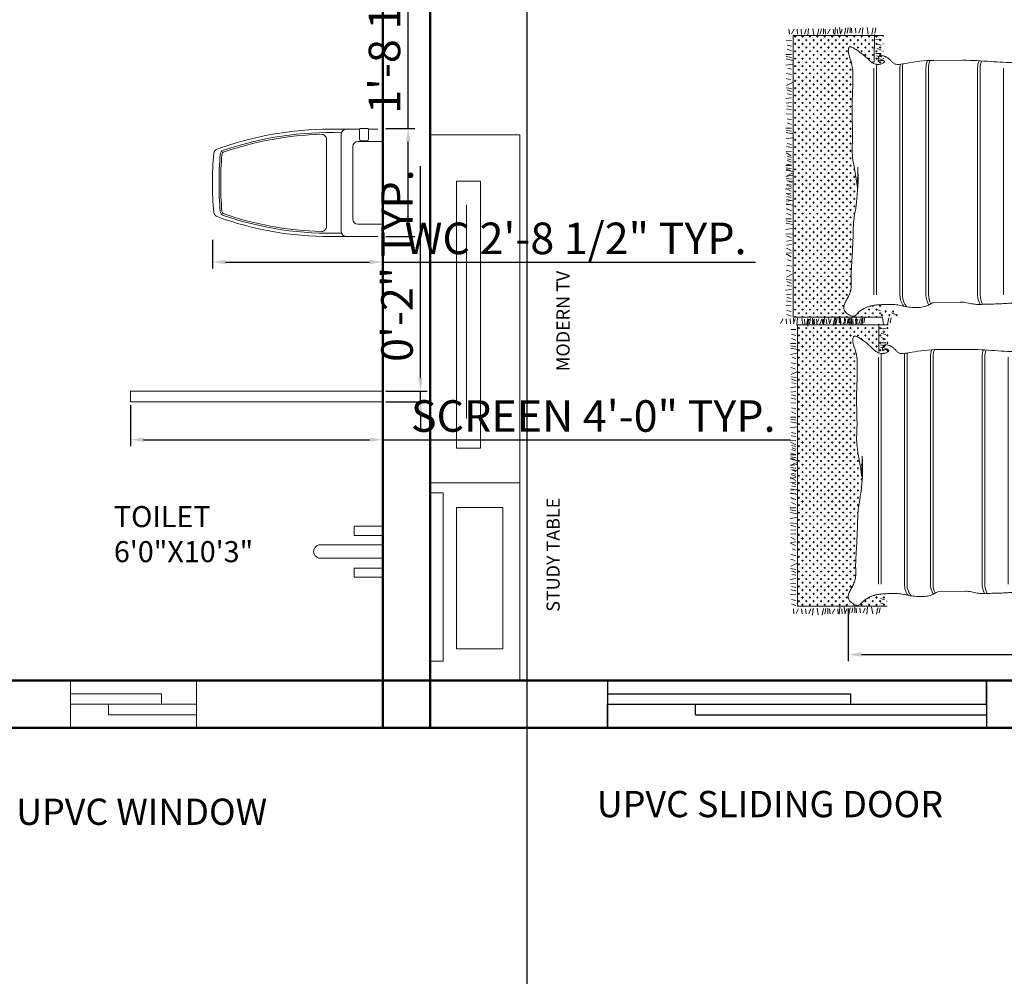
# Model space of a CAD drawing. Units: inches. Extents: x 2123 to 2977, y 1464 to 2698.
# Tile 3 of 10: x 2459 to 2647, y 1923 to 2105. Entities that reach past the tile are written whole.
import ezdxf

# ---------------------------------------------------------------- set-up
doc = ezdxf.new("R2010")
doc.units = ezdxf.units.IN
for name, color, linetype, lineweight in [('A-ANNO-DIMS', 2, 'Continuous', 18), ('A-ANNO-TEXT', 7, 'Continuous', 18), ('A-AREA-IDEN', 7, 'Continuous', 25), ('A-DOOR', 4, 'Continuous', 25), ('A-FLOR-FIXT', 8, 'Continuous', 20), ('A-FURN', 8, 'Continuous', 18), ('A-FURN-FIXD', 8, 'Continuous', 20), ('A-FURN-PATT', 252, 'Continuous', 9), ('A-GLAZ', 4, 'Continuous', 18), ('A-WALL', 7, 'Continuous', 50)]:
    doc.layers.add(name, color=color, linetype=linetype, lineweight=lineweight)
doc.styles.get("Standard").update_dxf_attribs({"font": 'arial.ttf'})
doc.dimstyles.new('ISO-25', dxfattribs={"dimtxt": 6, "dimasz": 2.5, "dimexe": 1.25, "dimexo": 0.625, "dimtad": 1, "dimdec": 0, "dimlunit": 3, "dimtxsty": 'Standard', "dimcen": 2.5, "dimadec": 0, "dimazin": 0, "dimtfac": 1, "dimtdec": 0, "dimtmove": 0, "dimatfit": 3, "dimfxl": 1, "dimarcsym": 0})

# ---------------------------------------------------------------- blocks, each defined once
blk = doc.blocks.new('WC-PLAN')
for p, q in [((27.97, 20.42), (22.38, 20.42)), ((24.5, 19.48), (24.5, 10.21)), ((27.93, 20.26), (27.93, 18.53)), ((29.37, 20.57), (28.24, 20.57)), ((31.41, 20.42), (29.65, 20.42)), ((29.69, 20.26), (29.69, 18.53)), ((32.35, 19.48), (32.35, 10.21)), ((21.67, 18.51), (21.67, 10.21)), ((26.7, 17.12), (26.7, 10.21)), ((32.35, 18.06), (27.64, 18.06)), ((29.37, 18.22), (28.24, 18.22)), ((28.24, 18.22), (28.24, 18.06)), ((29.37, 18.22), (29.37, 18.06)), ((21.67, 1.91), (21.67, 10.21)), ((24.5, 0.94), (24.5, 10.21)), ((26.7, 3.3), (26.7, 10.21)), ((32.35, 0.94), (32.35, 10.21)), ((32.35, 2.36), (27.64, 2.36)), ((31.41, 0), (22.38, 0))]:
    blk.add_line(p, q)
for centre, radius, start, end in [((22.38, -42.41), 62.82, 90, 110.0218), ((22.38, -42.41), 62.2, 88.0034, 109.0034), ((22.38, -42.41), 61.88, 91.5459, 109.0034), ((20.73, 18.51), 0.942, 0, 91.5459), ((25.44, 19.48), 0.942, 90, 180), ((28.24, 20.26), 0.314, 150, 180), ((28.24, 20.26), 0.314, 90, 150), ((29.37, 20.26), 0.314, 30, 90), ((29.37, 20.26), 0.314, 0, 30), ((27.64, 17.12), 0.942, 90, 180), ((28.24, 18.53), 0.314, 180, 270), ((29.37, 18.53), 0.314, 270, 0), ((62.98, 10.21), 62.98, 174.8892, 180), ((1.19, 15.74), 0.942, 110.0218, 174.8892), ((62.98, 10.21), 61.73, 174.9977, 180), ((2.43, 15.51), 0.942, 109.0034, 174.9977), ((62.98, 10.21), 61.41, 174.9977, 180), ((2.43, 15.51), 0.628, 109.0034, 174.9977), ((62.98, 10.21), 62.98, 180, 185.1108), ((62.98, 10.21), 61.73, 180, 185.0023), ((62.98, 10.21), 61.41, 180, 185.0023), ((1.19, 4.68), 0.942, 185.1108, 249.9782), ((22.38, 62.82), 62.82, 249.9782, 270), ((2.43, 4.91), 0.942, 185.0023, 250.9966), ((2.43, 4.91), 0.628, 185.0023, 250.9966), ((22.38, 62.82), 62.2, 250.9966, 271.9966), ((22.38, 62.82), 61.88, 250.9966, 268.4541), ((20.73, 1.91), 0.942, 268.4541, 0), ((27.64, 3.3), 0.942, 180, 270), ((25.44, 0.94), 0.942, 180, 270)]:
    blk.add_arc(centre, radius, start, end)
blk = doc.blocks.new('SHOWER-FITTING')
for points in [[(7.7, 9.7), (13.11, 9.7), (13.11, 7.96), (7.7, 7.96)], [(7.7, 1.74), (13.11, 1.74), (13.11, 0), (7.7, 0)]]:
    blk.add_lwpolyline(points, close=True)
blk.add_lwpolyline([(1, 6.13), (13.11, 6.13), (13.11, 3.63), (1, 3.63)])
blk.add_arc((1.29, 4.88), 1.29, 102.8146, 257.1854)
blk = doc.blocks.new('BED-WITH-PILLOWS')
for p, q in [((5.75, 4.05), (5.75, 47.2)), ((6.24, 4.05), (6.24, 47.2)), ((10.69, 4.05), (10.69, 47.2)), ((11.18, 4.05), (11.18, 47.2)), ((15.63, 4.05), (15.63, 47.2)), ((16.12, 4.05), (16.12, 47.2)), ((25.45, 4.05), (25.45, 47.2)), ((25.94, 4.05), (25.94, 47.2)), ((30.39, 4.05), (30.39, 47.2)), ((33.11, 4.05), (33.11, 47.2)), ((45.27, 2.11), (45.27, 48.58)), ((51.57, 46.51), (45.27, 46.51)), ((51.57, 45.27), (45.27, 45.27)), ((62.41, 46.17), (51.57, 46.17)), ((62.41, 45.03), (51.57, 45.03)), ((51.57, 28.22), (45.27, 28.22)), ((62.41, 5.26), (51.57, 5.26)), ((62.41, 4.13), (51.57, 4.13)), ((62.41, 2.86), (51.57, 2.86))]:
    blk.add_line(p, q)
for points in [[(51.2, 2.51), (50.14, 2.47), (49.31, 2.46), (48.67, 2.48), (48.19, 2.52), (47.84, 2.56), (47.58, 2.61), (47.39, 2.66), (47.22, 2.69), (47.07, 2.7), (46.91, 2.7), (46.77, 2.68), (46.63, 2.65), (46.51, 2.61), (46.41, 2.56), (46.33, 2.52), (46.28, 2.47), (46.26, 2.42), (46.26, 2.38), (46.28, 2.35), (46.3, 2.31), (46.32, 2.28), (46.32, 2.25), (46.31, 2.22), (46.27, 2.2), (46.19, 2.17), (46.08, 2.15), (45.94, 2.13), (45.78, 2.12), (45.61, 2.11), (45.43, 2.1), (45.25, 2.11), (45.07, 2.12), (44.89, 2.14), (44.73, 2.16), (44.57, 2.2), (44.42, 2.24), (44.28, 2.28), (44.15, 2.32), (44.02, 2.37), (43.89, 2.41), (43.77, 2.46), (43.65, 2.5), (43.51, 2.54), (43.35, 2.58), (43.16, 2.62), (42.93, 2.66), (42.65, 2.69), (42.31, 2.72), (41.91, 2.75), (41.46, 2.78), (40.97, 2.8), (40.46, 2.82), (39.94, 2.82), (39.43, 2.83), (38.94, 2.82), (38.48, 2.81), (38.08, 2.78), (37.71, 2.75), (37.37, 2.71), (37.04, 2.67), (36.71, 2.63), (36.37, 2.59), (36, 2.55), (35.6, 2.52), (35.14, 2.5), (34.65, 2.49), (34.14, 2.48), (33.61, 2.47), (33.1, 2.47), (32.6, 2.47), (32.14, 2.47), (31.72, 2.47), (31.37, 2.46), (31.06, 2.45), (30.79, 2.44), (30.55, 2.42), (30.31, 2.41), (30.08, 2.39), (29.82, 2.38), (29.54, 2.36), (29.21, 2.35), (28.86, 2.33), (28.48, 2.32), (28.09, 2.31), (27.69, 2.3), (27.3, 2.29), (26.93, 2.28), (26.58, 2.27), (26.27, 2.26), (25.99, 2.25), (25.73, 2.24), (25.49, 2.24), (25.25, 2.25), (25.02, 2.27), (24.78, 2.29), (24.53, 2.33), (24.27, 2.38), (23.99, 2.44), (23.7, 2.51), (23.41, 2.57), (23.12, 2.62), (22.85, 2.66), (22.59, 2.69), (22.35, 2.68), (22.13, 2.65), (17.06, 2.6), (16.88, 2.53), (16.71, 2.44), (16.54, 2.35), (16.37, 2.25), (16.2, 2.15), (16.01, 2.05), (15.8, 1.96), (15.58, 1.89), (15.34, 1.82), (15.08, 1.77), (14.81, 1.72), (14.53, 1.69), (14.24, 1.67), (13.93, 1.66), (13.62, 1.66), (13.3, 1.67), (12.98, 1.69), (12.67, 1.72), (12.35, 1.75), (12.05, 1.79), (11.76, 1.84), (11.49, 1.89), (11.24, 1.94), (11, 1.99), (10.76, 2.04), (10.52, 2.09), (10.28, 2.14), (10.02, 2.18), (9.74, 2.21), (9.43, 2.24), (9.08, 2.25), (8.71, 2.26), (8.32, 2.26), (7.93, 2.25), (7.53, 2.24), (7.16, 2.22), (6.8, 2.2), (6.49, 2.17), (6.21, 2.15), (5.97, 2.12), (5.77, 2.09), (5.59, 2.06), (5.44, 2.03), (5.3, 2), (5.18, 1.97), (5.07, 1.94), (4.96, 1.91), (4.85, 1.88), (4.74, 1.85), (4.63, 1.81), (4.51, 1.77), (4.39, 1.72), (4.26, 1.67), (4.12, 1.61), (3.98, 1.53), (3.82, 1.46), (3.67, 1.37), (3.51, 1.27), (3.35, 1.17), (3.19, 1.06), (3.04, 0.94), (2.9, 0.81), (2.76, 0.68), (2.64, 0.54), (2.52, 0.41), (2.4, 0.28), (2.28, 0.18), (2.15, 0.09), (2, 0.03), (1.84, 0), (1.67, 0.01), (1.48, 0.05), (1.28, 0.12), (1.09, 0.21), (0.89, 0.33), (0.71, 0.46), (0.54, 0.6), (0.39, 0.74), (0.26, 0.89), (0.17, 1.04), (0.09, 1.19), (0.04, 1.34), (0.01, 1.49), (0, 1.65), (0.01, 1.81), (0.04, 1.97), (0.08, 2.13), (0.14, 2.3), (0.21, 2.47), (0.29, 2.64), (0.38, 2.82), (0.48, 3), (0.58, 3.18), (0.68, 3.37), (0.79, 3.57), (0.9, 3.77), (1, 3.97), (1.09, 4.19), (1.18, 4.41), (1.26, 4.64), (1.32, 4.89), (1.37, 5.14), (1.4, 5.4), (1.42, 5.68), (1.43, 5.97), (1.43, 6.29), (1.42, 6.62), (1.42, 6.98), (1.41, 7.36), (1.41, 7.77), (1.42, 8.21), (1.44, 8.67), (1.46, 9.16), (1.49, 9.65), (1.52, 10.16), (1.55, 10.68), (1.58, 11.19), (1.61, 11.69), (1.64, 12.19), (1.67, 12.67), (1.69, 13.14), (1.72, 13.6), (1.73, 14.05), (1.75, 14.49), (1.77, 14.91), (1.78, 15.32), (1.79, 15.72), (1.79, 16.1), (1.8, 16.48), (1.81, 16.85), (1.83, 17.21), (1.85, 17.56), (1.88, 17.91), (1.91, 18.25), (1.96, 18.58), (2.01, 18.93), (2.07, 19.29), (2.14, 19.68), (2.21, 20.11), (2.29, 20.58), (2.36, 21.11), (2.44, 21.71), (2.51, 22.39), (2.58, 23.13), (2.64, 23.92), (2.69, 24.77), (2.72, 25.64), (2.73, 26.54), (2.71, 27.44), (2.67, 28.35), (2.59, 24.41), (2.49, 25.28), (2.37, 26.12), (2.24, 26.93), (2.11, 27.7), (1.98, 28.42), (1.86, 29.08), (1.76, 29.68), (1.69, 30.2), (1.64, 30.67), (1.61, 31.08), (1.59, 31.44), (1.59, 31.77), (1.6, 32.08), (1.61, 32.36), (1.63, 32.64), (1.64, 32.92), (1.66, 33.21), (1.67, 33.51), (1.67, 33.82), (1.68, 34.16), (1.68, 34.52), (1.68, 34.92), (1.67, 35.35), (1.66, 35.83), (1.64, 36.35), (1.62, 36.91), (1.61, 37.51), (1.6, 38.16), (1.59, 38.85), (1.59, 39.57), (1.6, 40.34), (1.62, 41.15), (1.65, 41.98), (1.68, 42.82), (1.7, 43.65), (1.72, 44.46), (1.73, 45.24), (1.72, 45.95), (1.7, 46.6), (1.64, 47.17), (1.57, 47.65), (1.48, 48.08), (1.39, 48.45), (1.29, 48.77), (1.19, 49.06), (1.1, 49.32), (1.02, 49.57), (0.96, 49.81), (0.91, 50.04), (0.89, 50.26), (0.87, 50.46), (0.88, 50.65), (0.9, 50.81), (0.93, 50.95), (0.98, 51.06), (1.04, 51.14), (1.12, 51.2), (1.21, 51.22), (1.31, 51.22), (1.43, 51.19), (1.55, 51.15), (1.69, 51.09), (1.84, 51.01), (2.01, 50.92), (2.18, 50.81), (2.36, 50.7), (2.54, 50.57), (2.72, 50.45), (2.91, 50.31), (3.09, 50.18), (3.27, 50.04), (3.45, 49.9), (3.62, 49.77), (3.78, 49.63), (3.93, 49.5), (4.08, 49.37), (4.23, 49.24), (4.37, 49.11), (4.5, 48.99), (4.63, 48.86), (4.76, 48.74), (4.88, 48.62), (5.01, 48.5), (5.14, 48.4), (5.27, 48.3), (5.41, 48.2), (5.55, 48.12), (5.71, 48.05), (5.87, 48), (6.04, 47.95), (6.22, 47.92), (6.39, 47.9), (6.56, 47.89), (6.73, 47.9), (6.89, 47.92), (7.04, 47.96), (7.18, 48.01), (7.31, 48.07), (7.43, 48.13), (7.53, 48.2), (7.61, 48.27), (7.67, 48.33), (7.71, 48.39), (7.73, 48.44), (7.73, 48.49), (7.71, 48.52), (7.68, 48.55), (7.63, 48.58), (7.56, 48.6), (7.49, 48.61), (7.42, 48.62), (7.33, 48.63), (7.25, 48.64), (7.16, 48.64), (7.07, 48.64), (6.99, 48.63), (6.91, 48.62), (6.83, 48.6), (6.77, 48.58), (6.71, 48.55), (6.67, 48.52), (6.63, 48.5), (6.6, 48.47), (6.57, 48.46), (6.56, 48.46), (6.55, 48.48), (6.54, 48.51), (6.54, 48.58)], [(6.54, 48.66), (6.54, 48.76), (6.55, 48.86), (6.56, 48.97), (6.58, 49.08), (6.61, 49.18), (6.63, 49.27), (6.67, 49.34), (6.7, 49.4), (6.75, 49.44), (6.79, 49.47), (6.84, 49.5), (6.9, 49.51), (6.95, 49.52), (7.01, 49.53), (7.07, 49.53), (7.14, 49.53), (7.21, 49.53), (7.28, 49.53), (7.35, 49.53), (7.43, 49.52), (7.51, 49.5), (7.59, 49.49), (7.68, 49.46), (7.77, 49.43), (7.86, 49.4), (7.96, 49.36), (8.06, 49.31), (8.16, 49.26), (8.27, 49.19), (8.37, 49.12), (8.48, 49.04), (8.59, 48.95), (8.69, 48.86), (8.8, 48.76), (8.9, 48.66), (9.01, 48.56), (9.1, 48.45), (9.2, 48.35), (9.29, 48.25), (9.38, 48.16), (9.48, 48.07), (9.61, 48), (9.76, 47.94), (9.95, 47.91), (10.18, 47.89), (10.46, 47.89), (10.81, 47.93), (11.21, 47.98), (11.65, 48.06), (12.15, 48.14), (12.68, 48.23), (13.25, 48.32), (13.84, 48.41), (14.46, 48.49), (15.09, 48.55), (15.74, 48.6), (16.41, 48.64), (17.08, 48.66), (22.63, 48.67), (23.31, 48.67), (23.98, 48.66), (24.65, 48.64), (25.32, 48.61), (25.97, 48.57), (26.62, 48.53), (27.26, 48.49), (27.89, 48.44), (28.51, 48.4), (29.12, 48.36), (29.71, 48.33), (30.3, 48.3), (30.87, 48.28), (31.43, 48.27), (31.97, 48.28), (32.5, 48.29), (33, 48.32), (33.49, 48.36), (33.95, 48.42), (34.39, 48.49), (34.81, 48.58), (35.23, 48.67), (35.64, 48.77), (36.07, 48.87), (36.5, 48.96), (36.96, 49.05), (37.46, 49.12), (37.99, 49.18), (38.55, 49.22), (39.13, 49.24), (39.73, 49.25), (40.33, 49.24), (40.93, 49.22), (41.52, 49.18), (42.1, 49.12), (42.65, 49.05), (43.17, 48.96), (43.66, 48.87), (44.14, 48.78), (44.58, 48.7), (45, 48.62), (45.4, 48.56), (45.77, 48.51), (46.12, 48.5), (46.45, 48.5), (46.77, 48.51), (47.08, 48.53), (47.4, 48.56), (47.73, 48.57), (48.08, 48.58), (48.45, 48.58), (48.84, 48.55), (49.25, 48.49), (49.68, 48.41), (50.1, 48.3), (50.5, 48.16), (50.88, 47.98), (51.23, 47.77), (51.53, 47.52)], [(51.57, 47.43), (51.57, 2.81), (45.27, 2.81)], [(51.57, 47.43), (62.41, 47.43)], [(45.27, 43.15), (51.57, 43.15)], [(51.57, 41.91), (45.27, 41.91)], [(45.27, 39.44), (51.57, 39.44)], [(51.57, 38.2), (45.27, 38.2)], [(45.27, 35.73), (51.57, 35.73)], [(51.57, 34.5), (45.27, 34.5)], [(45.27, 32.03), (51.57, 32.03)], [(51.57, 30.79), (45.27, 30.79)], [(45.27, 28.32), (51.57, 28.32)], [(51.57, 27.09), (45.27, 27.09)], [(45.27, 25.74), (51.57, 25.74)], [(45.27, 24.62), (51.57, 24.62)], [(51.57, 24.51), (45.27, 24.51)], [(51.57, 23.38), (45.27, 23.38)], [(45.27, 22.04), (51.57, 22.04)], [(51.57, 20.8), (45.27, 20.8)], [(45.27, 18.33), (51.57, 18.33)], [(51.57, 17.1), (45.27, 17.1)], [(45.27, 14.63), (51.57, 14.63)], [(51.57, 13.39), (45.27, 13.39)], [(45.27, 10.92), (51.57, 10.92)], [(51.57, 9.69), (45.27, 9.69)], [(45.27, 7.22), (51.57, 7.22)], [(51.57, 5.98), (45.27, 5.98)], [(45.27, 4.05), (51.57, 4.05)]]:
    blk.add_lwpolyline(points)
blk.add_lwpolyline([(51.57, 46.51), (51.57, 45.27), (45.27, 45.27), (45.27, 46.51)], close=True)
for centre, radius, start, end in [((9.74, 47.23), 3.5, 168.8455, 180.4575), ((14.19, 47.23), 3.5, 168.5644, 180.4575), ((14.68, 47.23), 3.5, 167.3874, 180.4575), ((19.13, 47.23), 3.5, 156.778, 180.4575), ((19.62, 47.23), 3.5, 156.3002, 180.4575), ((28.95, 47.23), 3.5, 157.2176, 180.4575), ((29.45, 47.23), 3.5, 157.7219, 180.4575), ((36.12, 47.23), 3.5, 162.3249, 180.4575), ((36.61, 47.23), 3.5, 162.5343, 180.4575), ((113.8, 36.55), 60.42, 176.9417, 187.4263), ((56.43, 21.05), 18.95, 81.0114, 98.9886), ((56.69, 54.69), 15.26, 257.8171, 275.8068), ((60.35, 32.94), 6.89, 82.0225, 107.8578), ((-19.09, 32.85), 80.7, 355.082, 4.918), ((33.93, 30.3), 20.02, 347.406, 13.4182), ((55.08, 36.57), 10.76, 261.3968, 285.5408), ((59.18, 20.45), 5.88, 68.7829, 101.9106), ((59.54, 25.52), 1.81, 13.0862, 85.1007), ((113.8, 22.01), 60.42, 176.9417, 187.4263), ((56.43, 6.52), 18.95, 81.0114, 98.9886), ((56.69, 40.15), 15.26, 257.8171, 275.8068), ((59.11, 48.58), 22.76, 264.4677, 275.5323), ((60.35, 18.41), 6.89, 82.0225, 107.8578), ((-19.09, 18.32), 80.7, 355.082, 4.918), ((33.93, 15.76), 20.02, 347.406, 13.4182), ((55.08, 22.03), 10.76, 261.3968, 285.5408), ((59.11, 34.05), 22.76, 264.4677, 275.5323), ((59.18, 5.91), 5.88, 68.7829, 101.9106), ((59.54, 10.99), 1.81, 13.0862, 85.1007), ((14.19, 4.02), 3.5, 179.5425, 217.0761), ((14.68, 4.02), 3.5, 179.5425, 219.1707), ((19.13, 4.02), 3.5, 179.5425, 212.5319), ((19.62, 4.02), 3.5, 179.5425, 208.4654), ((28.95, 4.02), 3.5, 179.5425, 210.3906), ((29.45, 4.02), 3.5, 179.5425, 210.1306), ((36.12, 4.02), 3.5, 179.5425, 206.8424), ((36.61, 4.02), 3.5, 179.5425, 206.471)]:
    blk.add_arc(centre, radius, start, end)
blk = doc.blocks.new('SHOWER-SCREEN')
for p, q in [((47.94, 2), (0, 2)), ((0, 2), (0, 0)), ((0, 0), (47.94, 0))]:
    blk.add_line(p, q)
blk = doc.blocks.new('*D42')
at = {"layer": 'A-ANNO-DIMS', "color": 0, "lineweight": -2, "transparency": 16777216}
for p, q in [((2496.08, 2062.68), (2496.08, 2057.2)), ((2528.44, 2062.68), (2528.44, 2057.2)), ((2498.58, 2058.45), (2525.94, 2058.45)), ((2528.44, 2058.45), (2599.28, 2058.45))]:
    blk.add_line(p, q, dxfattribs=at)
at = {"layer": 'A-ANNO-DIMS', "color": 0, "transparency": 16777216}
for points in [[(2498.58, 2058.87), (2498.58, 2058.03), (2496.08, 2058.45)], [(2525.94, 2058.87), (2525.94, 2058.03), (2528.44, 2058.45)]]:
    blk.add_solid(points, dxfattribs=at)
at = {"layer": 'Defpoints', "color": 0, "transparency": 16777216}
for p in [(2496.08, 2063.3), (2528.44, 2063.3), (2528.44, 2058.45)]:
    blk.add_point(p, dxfattribs=at)
at = {"layer": 'A-ANNO-DIMS', "color": 0, "transparency": 16777216, "insert": (2565.11, 2062.18), "char_height": 6, "attachment_point": 5}
blk.add_mtext('WC 2\'-8 1/2" TYP.', dxfattribs=at)
blk = doc.blocks.new('*D43')
at = {"layer": 'A-ANNO-DIMS', "color": 0, "lineweight": -2, "transparency": 16777216}
for p, q in [((2533.29, 2083.88), (2533.29, 2137.62)), ((2529.06, 2083.88), (2534.54, 2083.88)), ((2533.29, 2065.8), (2533.29, 2081.38)), ((2529.06, 2063.3), (2534.54, 2063.3))]:
    blk.add_line(p, q, dxfattribs=at)
at = {"layer": 'A-ANNO-DIMS', "color": 0, "transparency": 16777216}
for points in [[(2532.87, 2081.38), (2533.71, 2081.38), (2533.29, 2083.88)], [(2532.87, 2065.8), (2533.71, 2065.8), (2533.29, 2063.3)]]:
    blk.add_solid(points, dxfattribs=at)
at = {"layer": 'Defpoints', "color": 0, "transparency": 16777216}
for p in [(2528.44, 2083.88), (2533.29, 2083.88), (2528.44, 2063.3)]:
    blk.add_point(p, dxfattribs=at)
at = {"layer": 'A-ANNO-DIMS', "color": 0, "transparency": 16777216, "insert": (2529.56, 2112), "char_height": 6, "attachment_point": 5, "rotation": 90}
blk.add_mtext('1\'-8 1/2" TYP.', dxfattribs=at)
blk = doc.blocks.new('*D48')
at = {"layer": 'A-ANNO-DIMS', "color": 0, "lineweight": -2, "transparency": 16777216}
for p, q in [((2616.93, 1992.55), (2616.93, 1982.56)), ((2679.35, 1992.55), (2679.35, 1982.56)), ((2619.43, 1983.81), (2676.85, 1983.81)), ((2679.35, 1983.81), (2752.95, 1983.81))]:
    blk.add_line(p, q, dxfattribs=at)
at = {"layer": 'A-ANNO-DIMS', "color": 0, "transparency": 16777216}
for points in [[(2619.43, 1984.23), (2619.43, 1983.39), (2616.93, 1983.81)], [(2676.85, 1984.23), (2676.85, 1983.39), (2679.35, 1983.81)]]:
    blk.add_solid(points, dxfattribs=at)
at = {"layer": 'Defpoints', "color": 0, "transparency": 16777216}
for p in [(2616.93, 1993.17), (2679.35, 1993.17), (2679.35, 1983.81)]:
    blk.add_point(p, dxfattribs=at)
at = {"layer": 'A-ANNO-DIMS', "color": 0, "transparency": 16777216, "insert": (2717.4, 1987.54), "char_height": 6, "attachment_point": 5}
blk.add_mtext('BED 5\'-2 1/2" TYP.', dxfattribs=at)
blk = doc.blocks.new('*D52')
at = {"layer": 'A-ANNO-DIMS', "color": 0, "lineweight": -2, "transparency": 16777216}
for p, q in [((2480.5, 2031.24), (2480.5, 2023.42)), ((2528.44, 2031.24), (2528.44, 2023.42)), ((2483, 2024.67), (2525.94, 2024.67)), ((2528.44, 2024.67), (2605.99, 2024.67))]:
    blk.add_line(p, q, dxfattribs=at)
at = {"layer": 'A-ANNO-DIMS', "color": 0, "transparency": 16777216}
for points in [[(2483, 2025.09), (2483, 2024.26), (2480.5, 2024.67)], [(2525.94, 2025.09), (2525.94, 2024.26), (2528.44, 2024.67)]]:
    blk.add_solid(points, dxfattribs=at)
at = {"layer": 'Defpoints', "color": 0, "transparency": 16777216}
for p in [(2480.5, 2031.87), (2528.44, 2031.87), (2528.44, 2024.67)]:
    blk.add_point(p, dxfattribs=at)
at = {"layer": 'A-ANNO-DIMS', "color": 0, "transparency": 16777216, "insert": (2568.46, 2028.4), "char_height": 6, "attachment_point": 5}
blk.add_mtext('SCREEN 4\'-0" TYP.', dxfattribs=at)
blk = doc.blocks.new('*D53')
at = {"layer": 'A-ANNO-DIMS', "color": 0, "lineweight": -2, "transparency": 16777216}
for p, q in [((2535.63, 2036.37), (2535.63, 2076.69)), ((2529.06, 2033.87), (2536.88, 2033.87)), ((2535.63, 2031.87), (2535.63, 2033.87)), ((2529.06, 2031.87), (2536.88, 2031.87)), ((2535.63, 2029.37), (2535.63, 2026.87))]:
    blk.add_line(p, q, dxfattribs=at)
at = {"layer": 'A-ANNO-DIMS', "color": 0, "transparency": 16777216}
for points in [[(2535.21, 2036.37), (2536.04, 2036.37), (2535.63, 2033.87)], [(2535.21, 2029.37), (2536.04, 2029.37), (2535.63, 2031.87)]]:
    blk.add_solid(points, dxfattribs=at)
at = {"layer": 'Defpoints', "color": 0, "transparency": 16777216}
for p in [(2528.44, 2033.87), (2535.63, 2033.87), (2528.44, 2031.87)]:
    blk.add_point(p, dxfattribs=at)
at = {"layer": 'A-ANNO-DIMS', "color": 0, "transparency": 16777216, "insert": (2531.94, 2057.78), "char_height": 6, "attachment_point": 5, "rotation": 90}
blk.add_mtext('0\'-2" TYP.', dxfattribs=at)
blk = doc.blocks.new('*D57')
at = {"layer": 'A-ANNO-DIMS', "color": 0, "lineweight": -2, "transparency": 16777216}
for p, q in [((2555.89, 1805.13), (2555.89, 2606.82)), ((2558.39, 2605.57), (2755.44, 2605.57)), ((2757.94, 1805.13), (2757.94, 2606.82))]:
    blk.add_line(p, q, dxfattribs=at)
at = {"layer": 'A-ANNO-DIMS', "color": 0, "transparency": 16777216}
for points in [[(2558.39, 2605.99), (2558.39, 2605.15), (2555.89, 2605.57)], [(2755.44, 2605.99), (2755.44, 2605.15), (2757.94, 2605.57)]]:
    blk.add_solid(points, dxfattribs=at)
at = {"layer": 'Defpoints', "color": 0, "transparency": 16777216}
for p in [(2757.94, 2605.57), (2555.89, 1804.5), (2757.94, 1804.5)]:
    blk.add_point(p, dxfattribs=at)
at = {"layer": 'A-ANNO-DIMS', "color": 0, "transparency": 16777216, "insert": (2656.91, 2609.26), "char_height": 6, "attachment_point": 5}
blk.add_mtext('16\'-10"', dxfattribs=at)

msp = doc.modelspace()

# ---------------------------------------------------------------- hatches: boundary and pattern name
at = {"layer": 'A-FURN-PATT'}
h = msp.add_hatch(dxfattribs=at)
h.set_pattern_fill('CROSS', color=256, scale=0.1105279, style=0)
h.paths.add_polyline_path([(2606.45, 2047.98), (2623.47, 2047.98), (2623.47, 2050.38), (2623.23, 2050.37), (2622.28, 2050.3), (2621.66, 2050.22), (2621.26, 2050.13), (2620.92, 2050.03), (2620.59, 2049.92), (2620.2, 2049.76), (2619.74, 2049.52), (2619.26, 2049.21), (2618.84, 2048.83), (2618.48, 2048.44), (2618.08, 2048.18), (2617.56, 2048.2), (2616.97, 2048.48), (2616.46, 2048.9), (2616.17, 2049.34), (2616.08, 2049.81), (2616.15, 2050.29), (2616.36, 2050.79), (2616.65, 2051.34), (2616.97, 2051.92), (2617.26, 2052.57), (2617.45, 2053.29), (2617.5, 2054.13), (2617.49, 2055.13), (2617.5, 2056.36), (2617.56, 2057.81), (2617.66, 2059.34), (2617.75, 2060.83), (2617.81, 2062.2), (2617.85, 2063.47), (2617.88, 2064.64), (2617.92, 2065.71), (2618.03, 2066.74), (2618.21, 2067.84), (2618.44, 2069.27), (2618.66, 2071.28), (2618.79, 2073.8), (2618.74, 2076.5), (2618.45, 2074.28), (2618.05, 2076.57), (2617.77, 2078.36), (2617.67, 2079.6), (2617.69, 2080.52), (2617.73, 2081.36), (2617.75, 2082.31), (2617.74, 2083.51), (2617.7, 2085.06), (2617.67, 2087), (2617.7, 2089.3), (2617.78, 2091.81), (2617.8, 2094.11), (2617.65, 2095.81), (2617.36, 2096.92), (2617.1, 2097.72), (2616.96, 2098.41), (2616.97, 2098.97), (2617.12, 2099.3), (2617.39, 2099.37), (2617.77, 2099.24), (2618.25, 2098.97), (2618.8, 2098.6), (2619.35, 2098.19), (2619.85, 2097.79), (2620.3, 2097.4), (2620.71, 2097.02), (2621.08, 2096.66), (2621.48, 2096.36), (2621.95, 2096.15), (2622.47, 2096.05), (2622.97, 2096.08), (2623.39, 2096.22), (2623.65, 2096.4), (2623.65, 2101.52), (2606.45, 2101.52)])
h = msp.add_hatch(dxfattribs=at)
h.set_pattern_fill('CROSS', color=256, scale=0.1105279, style=0)
h.paths.add_polyline_path([(2607.31, 1993), (2624.33, 1993), (2624.33, 1995.4), (2624.09, 1995.39), (2623.14, 1995.32), (2622.52, 1995.23), (2622.11, 1995.14), (2621.78, 1995.05), (2621.44, 1994.94), (2621.06, 1994.78), (2620.6, 1994.54), (2620.12, 1994.23), (2619.7, 1993.85), (2619.33, 1993.46), (2618.94, 1993.2), (2618.41, 1993.22), (2617.82, 1993.5), (2617.32, 1993.91), (2617.02, 1994.36), (2616.93, 1994.82), (2617.01, 1995.3), (2617.22, 1995.81), (2617.51, 1996.35), (2617.83, 1996.94), (2618.11, 1997.58), (2618.3, 1998.31), (2618.36, 1999.15), (2618.35, 2000.15), (2618.35, 2001.38), (2618.42, 2002.83), (2618.52, 2004.36), (2618.6, 2005.84), (2618.67, 2007.22), (2618.71, 2008.49), (2618.74, 2009.65), (2618.78, 2010.73), (2618.89, 2011.76), (2619.07, 2012.85), (2619.29, 2014.28), (2619.51, 2016.3), (2619.65, 2018.81), (2619.6, 2021.52), (2619.3, 2019.29), (2618.91, 2021.59), (2618.62, 2023.37), (2618.53, 2024.61), (2618.55, 2025.54), (2618.59, 2026.38), (2618.61, 2027.33), (2618.6, 2028.52), (2618.56, 2030.08), (2618.52, 2032.02), (2618.55, 2034.32), (2618.64, 2036.82), (2618.66, 2039.12), (2618.5, 2040.83), (2618.22, 2041.94), (2617.95, 2042.74), (2617.82, 2043.43), (2617.83, 2043.98), (2617.98, 2044.32), (2618.24, 2044.39), (2618.63, 2044.26), (2619.11, 2043.98), (2619.66, 2043.62), (2620.21, 2043.21), (2620.71, 2042.81), (2621.16, 2042.41), (2621.56, 2042.03), (2621.94, 2041.68), (2622.34, 2041.38), (2622.81, 2041.17), (2623.32, 2041.07), (2623.82, 2041.09), (2624.25, 2041.24), (2624.51, 2041.41), (2624.51, 2046.54), (2607.31, 2046.54)])

# ---------------------------------------------------------------- linework, layer by layer
at = {"layer": 'A-DOOR'}
for p, q in [((2571.19, 1978.87), (2571.19, 1969.87)), ((2643.19, 1974.37), (2643.19, 1978.87)), ((2643.19, 1978.87), (2643.19, 1969.87)), ((2571.19, 1976.37), (2617.34, 1976.37)), ((2617.34, 1976.37), (2617.34, 1974.37)), ((2571.19, 1969.87), (2571.19, 1974.37)), ((2571.19, 1974.37), (2643.19, 1974.37)), ((2587.91, 1972.37), (2587.91, 1974.37)), ((2587.91, 1972.37), (2643.19, 1972.37))]:
    msp.add_line(p, q, dxfattribs=at)
at = {"layer": 'A-FURN'}
for p, q in [((2605.67, 2102.74), (2605.76, 2101.8)), ((2606.64, 2102.74), (2606.16, 2101.88)), ((2607.23, 2102.74), (2607.32, 2101.8)), ((2607.98, 2102.74), (2608.07, 2101.8)), ((2608.95, 2102.74), (2608.6, 2101.8)), ((2609.39, 2102.89), (2609.26, 2101.57)), ((2610.18, 2102.89), (2610.38, 2101.64)), ((2611.37, 2102.82), (2611.1, 2101.57)), ((2611.83, 2102.82), (2611.63, 2101.8)), ((2612.22, 2102.89), (2612.22, 2101.84)), ((2612.52, 2102.74), (2612.61, 2101.8)), ((2613.5, 2102.74), (2613.01, 2101.88)), ((2614.08, 2102.74), (2614.17, 2101.8)), ((2614.49, 2103.07), (2614.36, 2101.74)), ((2614.83, 2102.74), (2614.93, 2101.8)), ((2615.28, 2103.07), (2615.48, 2101.82)), ((2615.81, 2102.74), (2615.45, 2101.8)), ((2616.47, 2102.99), (2616.2, 2101.74)), ((2616.93, 2102.99), (2616.74, 2101.98)), ((2617.32, 2103.07), (2617.32, 2102.02)), ((2617.56, 2102.92), (2617.65, 2101.98)), ((2618.32, 2102.92), (2618.41, 2101.98)), ((2619.29, 2102.92), (2618.93, 2101.98)), ((2619.72, 2103.07), (2619.6, 2101.74)), ((2620.52, 2103.07), (2620.72, 2101.82)), ((2621.7, 2102.99), (2621.44, 2101.74)), ((2622.16, 2102.99), (2621.97, 2101.98)), ((2605.15, 2100.63), (2606.13, 2100.58)), ((2606.45, 2047.98), (2606.45, 2101.52)), ((2606.45, 2101.52), (2623.65, 2101.52)), ((2621.9, 2101.7), (2621.87, 2096.45)), ((2622.21, 2100.81), (2623.2, 2100.76)), ((2605.3, 2099.71), (2606.13, 2099.49)), ((2605.3, 2098.92), (2606.13, 2098.59)), ((2622.15, 2098.1), (2623.2, 2098.1)), ((2622.36, 2099.89), (2623.2, 2099.67)), ((2622.36, 2099.1), (2623.2, 2098.77)), ((2605.08, 2097.93), (2606.13, 2097.93)), ((2605.16, 2097.53), (2606.17, 2097.34)), ((2605.16, 2097.07), (2606.41, 2096.8)), ((2622.22, 2097.7), (2623.24, 2097.51)), ((2622.22, 2097.24), (2623.47, 2096.98)), ((2605.08, 2095.88), (2606.33, 2096.09)), ((2605.45, 2095.35), (2606.13, 2095.12)), ((2605.15, 2093.37), (2606.01, 2093.11)), ((2605.22, 2092.05), (2606.32, 2092.58)), ((2605.23, 2094.31), (2606.16, 2094.1)), ((2605.15, 2091.59), (2606.17, 2091.46)), ((2605.3, 2091.19), (2606.17, 2090.86)), ((2605.07, 2089.54), (2606.13, 2089.7)), ((2605.15, 2088.69), (2606.13, 2088.82)), ((2605.37, 2090.47), (2606.17, 2090.33)), ((2605.22, 2087.56), (2606.13, 2087.38)), ((2605.3, 2088.16), (2606.13, 2087.97)), ((2605.15, 2086.64), (2606.13, 2086.59)), ((2605.3, 2085.72), (2606.13, 2085.5)), ((2605.08, 2083.94), (2606.13, 2083.94)), ((2605.16, 2083.54), (2606.17, 2083.35)), ((2605.16, 2083.08), (2606.41, 2082.81)), ((2605.3, 2084.93), (2606.13, 2084.61)), ((2605.08, 2081.89), (2606.33, 2082.1)), ((2605.15, 2079.49), (2606.13, 2079.44)), ((2605.22, 2080.41), (2606.13, 2080.23)), ((2605.3, 2081.01), (2606.13, 2080.82)), ((2605.11, 2079.21), (2606.1, 2078.66)), ((2605.3, 2078.57), (2606.13, 2078.35)), ((2605.3, 2077.78), (2606.13, 2077.46)), ((2605.41, 2078.1), (2606.1, 2077.87)), ((2605.08, 2076.79), (2606.13, 2076.79)), ((2605.11, 2076.13), (2605.98, 2075.86)), ((2605.16, 2076.39), (2606.17, 2076.2)), ((2605.16, 2075.93), (2606.41, 2075.66)), ((2605.2, 2077.06), (2606.13, 2076.85)), ((2605.08, 2074.74), (2606.33, 2074.95)), ((2605.11, 2074.34), (2606.14, 2074.21)), ((2605.19, 2074.8), (2606.29, 2075.33)), ((2605.26, 2073.94), (2606.14, 2073.61)), ((2605.56, 2073.9), (2606.36, 2073.72)), ((2605.04, 2072.3), (2606.1, 2072.45)), ((2605.11, 2072.47), (2606.1, 2071.92)), ((2605.2, 2073.11), (2606.14, 2072.67)), ((2605.34, 2073.23), (2606.14, 2073.09)), ((2605.11, 2071.44), (2606.1, 2071.57)), ((2605.11, 2070.05), (2606.29, 2070.18)), ((2605.19, 2070.32), (2606.1, 2070.13)), ((2605.26, 2070.92), (2606.1, 2070.73)), ((2605.41, 2071.37), (2606.1, 2071.13)), ((2605.11, 2069.4), (2606.1, 2069.35)), ((2605.19, 2069.53), (2606.36, 2069.26)), ((2605.2, 2068.65), (2606.14, 2068.21)), ((2605.26, 2068.48), (2606.1, 2068.25)), ((2605.05, 2066.69), (2606.1, 2066.69)), ((2605.12, 2066.29), (2606.14, 2066.1)), ((2605.26, 2067.68), (2606.1, 2067.36)), ((2605.05, 2064.65), (2606.3, 2064.85)), ((2605.12, 2065.83), (2606.37, 2065.57)), ((2605.05, 2063.85), (2606.37, 2063.73)), ((2605.2, 2063.42), (2606.14, 2063.06)), ((2605.2, 2062.45), (2606.14, 2062.54)), ((2605.2, 2061.69), (2606.14, 2061.78)), ((2605.2, 2061.11), (2606.06, 2060.62)), ((2605.11, 2060), (2606.1, 2059.45)), ((2605.2, 2060.13), (2606.14, 2060.22)), ((2605.41, 2058.9), (2606.1, 2058.66)), ((2605.11, 2056.92), (2605.98, 2056.65)), ((2605.2, 2057.85), (2606.13, 2057.65)), ((2605.11, 2055.13), (2606.14, 2055)), ((2605.19, 2055.59), (2606.29, 2056.13)), ((2605.04, 2053.09), (2606.1, 2053.24)), ((2605.26, 2054.74), (2606.14, 2054.4)), ((2605.34, 2054.02), (2606.14, 2053.88)), ((2605.11, 2052.23), (2606.1, 2052.37)), ((2605.26, 2051.71), (2606.1, 2051.52)), ((2605.11, 2050.19), (2606.1, 2050.14)), ((2605.19, 2051.11), (2606.1, 2050.92)), ((2622.2, 2049.44), (2623.04, 2049.22)), ((2604.56, 2047.63), (2604.07, 2046.76)), ((2605.14, 2047.63), (2605.23, 2046.69)), ((2605.26, 2049.27), (2606.1, 2049.05)), ((2605.26, 2048.48), (2606.1, 2048.15)), ((2605.89, 2047.63), (2605.98, 2046.69)), ((2623.47, 2047.98), (2606.45, 2047.98)), ((2606.87, 2047.63), (2606.51, 2046.69)), ((2606.52, 2047.76), (2606.62, 2046.82)), ((2607.3, 2047.78), (2607.17, 2046.45)), ((2608.09, 2047.78), (2608.29, 2046.53)), ((2608.61, 2047.6), (2608.7, 2046.66)), ((2609.28, 2047.7), (2609.01, 2046.45)), ((2609.59, 2047.6), (2609.1, 2046.73)), ((2609.39, 2047.62), (2609.26, 2046.29)), ((2609.74, 2047.7), (2609.55, 2046.69)), ((2610.13, 2047.78), (2610.13, 2046.73)), ((2610.17, 2047.6), (2610.26, 2046.66)), ((2610.18, 2047.62), (2610.38, 2046.37)), ((2610.43, 2047.63), (2610.52, 2046.69)), ((2611.41, 2047.63), (2610.92, 2046.76)), ((2610.93, 2047.6), (2611.02, 2046.66)), ((2611.9, 2047.6), (2611.54, 2046.66)), ((2611.99, 2047.63), (2612.08, 2046.69)), ((2612.22, 2047.62), (2612.22, 2046.57)), ((2612.4, 2047.95), (2612.27, 2046.63)), ((2612.75, 2047.63), (2612.84, 2046.69)), ((2613.19, 2047.95), (2613.4, 2046.7)), ((2613.72, 2047.63), (2613.36, 2046.69)), ((2614.31, 2047.67), (2614.05, 2046.42)), ((2614.38, 2047.88), (2614.11, 2046.63)), ((2614.49, 2047.79), (2614.36, 2046.47)), ((2614.77, 2047.67), (2614.58, 2046.66)), ((2614.84, 2047.88), (2614.65, 2046.86)), ((2615.24, 2047.95), (2615.24, 2046.9)), ((2615.28, 2047.79), (2615.48, 2046.54)), ((2615.47, 2047.8), (2615.56, 2046.86)), ((2615.47, 2047.6), (2615.56, 2046.66)), ((2616.45, 2047.6), (2615.96, 2046.73)), ((2616.47, 2047.72), (2616.2, 2046.47)), ((2616.23, 2047.8), (2616.32, 2046.86)), ((2616.93, 2047.72), (2616.74, 2046.7)), ((2617.2, 2047.8), (2616.84, 2046.86)), ((2617.03, 2047.6), (2617.12, 2046.66)), ((2617.32, 2047.79), (2617.32, 2046.74)), ((2617.64, 2047.95), (2617.51, 2046.63)), ((2617.56, 2047.64), (2617.65, 2046.7)), ((2617.78, 2047.6), (2617.87, 2046.66)), ((2618.32, 2047.64), (2618.41, 2046.7)), ((2618.76, 2047.6), (2618.4, 2046.66)), ((2618.43, 2047.95), (2618.63, 2046.7)), ((2619.29, 2047.64), (2618.93, 2046.7)), ((2619.61, 2047.88), (2619.35, 2046.63)), ((2619.72, 2047.79), (2619.6, 2046.47)), ((2620.07, 2047.88), (2619.88, 2046.86)), ((2623.17, 2048.36), (2623.52, 2048.36)), ((2623.34, 2048.18), (2623.34, 2048.53)), ((2623.46, 2047.92), (2623.67, 2046.67)), ((2623.87, 2049.06), (2624.22, 2049.06)), ((2624.04, 2048.88), (2624.04, 2049.24)), ((2624.65, 2047.85), (2624.38, 2046.6)), ((2624.57, 2048.36), (2624.92, 2048.36)), ((2624.75, 2048.18), (2624.75, 2048.53)), ((2625.11, 2047.85), (2624.92, 2046.83)), ((2625.15, 2048.79), (2625.98, 2048.46)), ((2625.27, 2049.06), (2625.62, 2049.06)), ((2625.45, 2048.88), (2625.45, 2049.24)), ((2625.97, 2048.36), (2626.33, 2048.36)), ((2626.15, 2048.18), (2626.15, 2048.53)), ((2606.01, 2045.65), (2606.99, 2045.6)), ((2607.31, 1993), (2607.31, 2046.54)), ((2607.31, 2046.54), (2624.51, 2046.54)), ((2622.76, 2046.71), (2622.73, 2041.47)), ((2623.07, 2045.82), (2624.06, 2045.77)), ((2606.16, 2044.73), (2606.99, 2044.51)), ((2606.16, 2043.94), (2606.99, 2043.61)), ((2623.22, 2044.9), (2624.06, 2044.68)), ((2623.22, 2044.11), (2624.06, 2043.79)), ((2605.94, 2042.94), (2606.99, 2042.94)), ((2606.02, 2042.55), (2607.03, 2042.35)), ((2606.02, 2042.09), (2607.27, 2041.82)), ((2623.01, 2043.12), (2624.06, 2043.12)), ((2623.08, 2042.72), (2624.1, 2042.53)), ((2623.08, 2042.26), (2624.33, 2041.99)), ((2605.94, 2040.9), (2607.19, 2041.1)), ((2606.3, 2040.37), (2606.99, 2040.13)), ((2606.01, 2038.39), (2606.87, 2038.12)), ((2606.09, 2039.32), (2607.02, 2039.12)), ((2606.01, 2036.6), (2607.03, 2036.48)), ((2606.08, 2037.06), (2607.18, 2037.6)), ((2605.93, 2034.56), (2606.99, 2034.71)), ((2606.16, 2036.21), (2607.03, 2035.88)), ((2606.23, 2035.49), (2607.03, 2035.35)), ((2606.01, 2033.7), (2606.99, 2033.84)), ((2606.08, 2032.58), (2606.99, 2032.39)), ((2606.16, 2033.18), (2606.99, 2032.99)), ((2606.01, 2031.66), (2606.99, 2031.61)), ((2606.16, 2030.74), (2606.99, 2030.52)), ((2605.94, 2028.95), (2606.99, 2028.95)), ((2606.16, 2029.95), (2606.99, 2029.62)), ((2605.94, 2026.91), (2607.19, 2027.11)), ((2606.02, 2028.56), (2607.03, 2028.37)), ((2606.02, 2028.1), (2607.27, 2027.83)), ((2606.08, 2025.43), (2606.99, 2025.25)), ((2606.16, 2026.03), (2606.99, 2025.84)), ((2605.97, 2024.22), (2606.95, 2023.67)), ((2606.01, 2024.51), (2606.99, 2024.46)), ((2606.16, 2023.59), (2606.99, 2023.37)), ((2605.94, 2021.81), (2606.99, 2021.81)), ((2606.02, 2021.41), (2607.03, 2021.22)), ((2606.05, 2022.08), (2606.98, 2021.87)), ((2606.16, 2022.8), (2606.99, 2022.47)), ((2606.27, 2023.12), (2606.95, 2022.88)), ((2605.94, 2019.76), (2607.19, 2019.97)), ((2605.97, 2021.14), (2606.83, 2020.88)), ((2606.02, 2020.95), (2607.27, 2020.68)), ((2606.04, 2019.82), (2607.14, 2020.35)), ((2605.97, 2019.36), (2606.99, 2019.23)), ((2606.05, 2018.13), (2606.99, 2017.69)), ((2606.12, 2018.96), (2606.99, 2018.63)), ((2606.19, 2018.24), (2606.99, 2018.1)), ((2606.42, 2018.92), (2607.22, 2018.74)), ((2605.89, 2017.31), (2606.95, 2017.47)), ((2605.97, 2017.49), (2606.95, 2016.94)), ((2605.97, 2016.46), (2606.95, 2016.59)), ((2606.12, 2015.93), (2606.95, 2015.74)), ((2606.27, 2016.38), (2606.95, 2016.15)), ((2605.97, 2015.07), (2607.14, 2015.2)), ((2605.97, 2014.41), (2606.95, 2014.36)), ((2606.04, 2015.33), (2606.95, 2015.15)), ((2606.04, 2014.55), (2607.22, 2014.28)), ((2606.05, 2013.67), (2606.99, 2013.23)), ((2606.12, 2013.49), (2606.95, 2013.27)), ((2606.12, 2012.7), (2606.95, 2012.37)), ((2605.9, 2011.71), (2606.95, 2011.71)), ((2605.98, 2011.31), (2606.99, 2011.12)), ((2605.98, 2010.85), (2607.23, 2010.58)), ((2605.9, 2009.66), (2607.15, 2009.87)), ((2605.9, 2008.87), (2607.23, 2008.74)), ((2606.05, 2008.44), (2606.99, 2008.08)), ((2606.05, 2007.46), (2606.99, 2007.56)), ((2606.05, 2006.71), (2606.99, 2006.8)), ((2605.97, 2005.02), (2606.95, 2004.47)), ((2606.05, 2006.13), (2606.92, 2005.64)), ((2606.05, 2005.15), (2606.99, 2005.24)), ((2606.05, 2002.87), (2606.98, 2002.67)), ((2606.27, 2003.92), (2606.95, 2003.68)), ((2605.97, 2001.94), (2606.83, 2001.67)), ((2606.04, 2000.61), (2607.14, 2001.14)), ((2605.97, 2000.15), (2606.99, 2000.02)), ((2606.12, 1999.75), (2606.99, 1999.42)), ((2606.19, 1999.04), (2606.99, 1998.9)), ((2605.89, 1998.11), (2606.95, 1998.26)), ((2605.97, 1997.25), (2606.95, 1997.39)), ((2605.97, 1995.21), (2606.95, 1995.16)), ((2606.04, 1996.13), (2606.95, 1995.94)), ((2606.12, 1996.73), (2606.95, 1996.54)), ((2606.12, 1994.29), (2606.95, 1994.07)), ((2606.12, 1993.49), (2606.95, 1993.17)), ((2623.06, 1994.46), (2623.89, 1994.24)), ((2623.06, 1993.67), (2623.89, 1993.34)), ((2606.52, 1992.48), (2606.62, 1991.54)), ((2607.5, 1992.48), (2607.01, 1991.62)), ((2624.33, 1993), (2607.31, 1993)), ((2608.08, 1992.48), (2608.17, 1991.54)), ((2608.84, 1992.48), (2608.93, 1991.54)), ((2609.81, 1992.48), (2609.45, 1991.54)), ((2610.25, 1992.63), (2610.12, 1991.31)), ((2611.04, 1992.63), (2611.24, 1991.38)), ((2612.22, 1992.56), (2611.96, 1991.31)), ((2612.68, 1992.56), (2612.49, 1991.54)), ((2613.08, 1992.63), (2613.08, 1991.58)), ((2613.38, 1992.48), (2613.47, 1991.54)), ((2614.36, 1992.48), (2613.87, 1991.62)), ((2614.94, 1992.48), (2615.03, 1991.54)), ((2615.35, 1992.81), (2615.22, 1991.48)), ((2615.69, 1992.48), (2615.78, 1991.54)), ((2616.14, 1992.81), (2616.34, 1991.56)), ((2616.67, 1992.48), (2616.31, 1991.54)), ((2617.33, 1992.73), (2617.06, 1991.48)), ((2617.79, 1992.73), (2617.59, 1991.72)), ((2618.18, 1992.81), (2618.18, 1991.76)), ((2618.42, 1992.66), (2618.51, 1991.72)), ((2619.17, 1992.66), (2619.27, 1991.72)), ((2620.15, 1992.66), (2619.79, 1991.72)), ((2620.58, 1992.81), (2620.45, 1991.48)), ((2621.37, 1992.81), (2621.58, 1991.56)), ((2622.56, 1992.73), (2622.29, 1991.48)), ((2623.02, 1992.73), (2622.83, 1991.72))]:
    msp.add_line(p, q, dxfattribs=at)
at = {"layer": 'A-FURN-FIXD'}
for p, q in [((2544.35, 2069.34), (2544.35, 2028.7)), ((2537.44, 2016.47), (2554.52, 2016.47))]:
    msp.add_line(p, q, dxfattribs=at)
for points in [[(2537.44, 2082.63), (2554.52, 2082.63), (2554.52, 1978.87), (2537.44, 1978.87)], [(2547.05, 2073.83), (2542.5, 2073.83), (2542.5, 2023.05), (2547.05, 2023.05)], [(2537.44, 2014.55), (2539.92, 2014.55), (2539.92, 1982.55), (2537.44, 1982.55)], [(2542.5, 2011.8), (2551.25, 2011.8), (2551.25, 1984.89), (2542.5, 1984.89)]]:
    msp.add_lwpolyline(points, close=True, dxfattribs=at)
at = {"layer": 'A-GLAZ'}
for p, q in [((2469.08, 1978.87), (2469.08, 1969.87)), ((2493.08, 1974.37), (2493.08, 1978.87)), ((2493.08, 1978.87), (2493.08, 1969.87)), ((2469.08, 1976.37), (2486.41, 1976.37)), ((2486.41, 1976.37), (2486.41, 1974.37)), ((2469.08, 1969.87), (2469.08, 1974.37)), ((2469.08, 1974.37), (2493.08, 1974.37)), ((2476.3, 1974.37), (2476.3, 1972.37)), ((2476.3, 1972.37), (2493.08, 1972.37))]:
    msp.add_line(p, q, dxfattribs=at)
at = {"layer": 'A-WALL'}
for p, q in [((2528.44, 2155.87), (2528.44, 1969.87)), ((2528.44, 2155.87), (2528.44, 1969.87)), ((2537.44, 2155.87), (2537.44, 1969.87)), ((2528.44, 2042.7), (2528.44, 2104.32)), ((2456.44, 1978.87), (2685.94, 1978.87)), ((2447.44, 1969.87), (2685.94, 1969.87))]:
    msp.add_line(p, q, dxfattribs=at)

# ---------------------------------------------------------------- block references
at = {"layer": 'A-FLOR-FIXT'}
for name, p in [('WC-PLAN', (2496.08, 2063.3)), ('SHOWER-SCREEN', (2480.5, 2031.87)), ('SHOWER-FITTING', (2515.32, 1998.52))]:
    msp.add_blockref(name, p, dxfattribs=at)
at = {"layer": 'A-FURN'}
for p in [(2616.08, 2048.15), (2616.93, 1993.17)]:
    msp.add_blockref('BED-WITH-PILLOWS', p, dxfattribs=at)

# ---------------------------------------------------------------- texts
at = {"layer": 'A-ANNO-TEXT', "char_height": 2.5, "attachment_point": 1, "rotation": 90}
for s, width, insert in [('MODERN TV', 114.4728, (2561.47, 2037.71)), ('STUDY TABLE', 247.9493, (2559.59, 1991.96))]:
    msp.add_mtext_dynamic_manual_height_columns(s, width=width, gutter_width=12.5, heights=[0], dxfattribs=dict(at, insert=insert))
at = {"layer": 'A-ANNO-TEXT', "char_height": 5, "attachment_point": 1}
for s, width, insert in [('UPVC SLIDING DOOR', 154.7653, (2569.15, 1957.88)), ('UPVC WINDOW', 103.2245, (2458.78, 1956.42))]:
    msp.add_mtext_dynamic_manual_height_columns(s, width=width, gutter_width=12.5, heights=[0], dxfattribs=dict(at, insert=insert))
at = {"layer": 'A-AREA-IDEN', "insert": (2477.35, 2012.05), "char_height": 4, "attachment_point": 1}
msp.add_mtext_dynamic_manual_height_columns('TOILET\\P6\'0"X10\'3"', width=166.3871, gutter_width=12.5, heights=[0], dxfattribs=at)

# ---------------------------------------------------------------- dimensions: what is measured, and where the dimension line sits
at = {"layer": 'A-ANNO-DIMS'}
dim = msp.add_linear_dim(base=(2757.9353, 2605.5708), p1=(2555.8869, 1804.5032), p2=(2757.9353, 1804.5032), dimstyle='ISO-25', override={"dimdec": 1, "dimlfac": 1, "dimrnd": 0, "dimzin": 1, "dimdsep": 46, "dimlunit": 4, "dimfrac": 2}, dxfattribs=at)
dim.commit()
dim.dimension.update_dxf_attribs({"geometry": '*D57', "text_midpoint": (2656.9111, 2609.2592)})
for base, p1, p2, picture, middle in [((2533.29, 2083.88), (2528.44, 2063.3), (2528.44, 2083.88), '*D43', (2529.56, 2112)), ((2535.63, 2033.87), (2528.44, 2031.87), (2528.44, 2033.87), '*D53', (2531.94, 2057.78))]:
    dim = msp.add_linear_dim(base=base, p1=p1, p2=p2, angle=90, text='<> TYP.', dimstyle='ISO-25', override={"dimdec": 1, "dimlfac": 1, "dimrnd": 0, "dimzin": 1, "dimdsep": 46, "dimlunit": 4, "dimfrac": 2}, dxfattribs=at)
    dim.commit()
    dim.dimension.update_dxf_attribs({"geometry": picture, "text_midpoint": middle})
for base, p1, p2, text, picture, middle in [((2528.44, 2058.45), (2496.08, 2063.3), (2528.44, 2063.3), 'WC <> TYP.', '*D42', (2565.11, 2062.18)), ((2528.44, 2024.67), (2480.5, 2031.87), (2528.44, 2031.87), 'SCREEN <> TYP.', '*D52', (2568.46, 2028.4)), ((2679.35, 1983.81), (2616.93, 1993.17), (2679.35, 1993.17), 'BED <> TYP.', '*D48', (2717.4, 1987.54))]:
    dim = msp.add_linear_dim(base=base, p1=p1, p2=p2, text=text, dimstyle='ISO-25', override={"dimdec": 1, "dimlfac": 1, "dimrnd": 0, "dimzin": 1, "dimdsep": 46, "dimlunit": 4, "dimfrac": 2}, dxfattribs=at)
    dim.commit()
    dim.dimension.update_dxf_attribs({"geometry": picture, "text_midpoint": middle})

doc.saveas('drawing.dxf')
